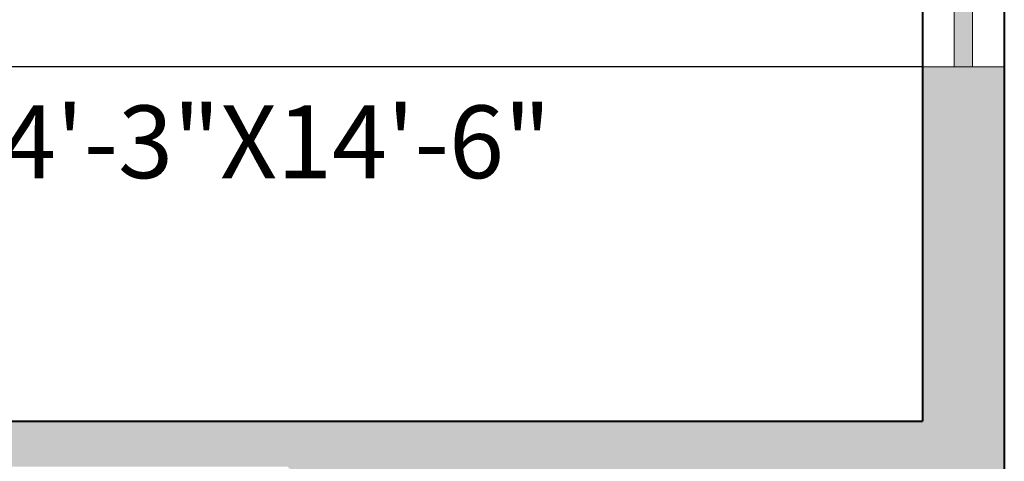
# Model space of a CAD drawing. Units: inches. Extents: x 2330 to 3943, y 1763 to 3461.
# Tile 32 of 40: x 3347 to 3456, y 2975 to 3024. Entities that reach past the tile are written whole.
import ezdxf

# ---------------------------------------------------------------- set-up
doc = ezdxf.new("R2010")
doc.units = ezdxf.units.IN
for name, color, linetype, lineweight in [('A-ANNO-DIMS', 2, 'Continuous', 18), ('A-AREA-IDEN', 7, 'Continuous', 18), ('A-GLAZ', 4, 'Continuous', 18), ('A-WALL', 7, 'Continuous', 40), ('A-WALL-PATT', 252, 'Continuous', 13)]:
    doc.layers.add(name, color=color, linetype=linetype, lineweight=lineweight)
doc.styles.get("Standard").update_dxf_attribs({"font": 'arial.ttf'})
doc.dimstyles.get("Standard").update_dxf_attribs({"dimtxt": 0.18, "dimasz": 0.18, "dimexe": 0.18, "dimexo": 0.0625, "dimgap": 0.09, "dimtad": 0, "dimtih": 1, "dimtoh": 1, "dimdec": 4, "dimzin": 0, "dimdsep": 46, "dimtxsty": 'Standard', "dimcen": 0.09, "dimadec": 0, "dimazin": 0, "dimtfac": 1, "dimtdec": 4, "dimtofl": 0, "dimtmove": 0, "dimatfit": 3, "dimfxl": 1, "dimtolj": 1, "dimtzin": 0, "dimarcsym": 0})

# ---------------------------------------------------------------- blocks, each defined once
blk = doc.blocks.new('WINDOW-96IN')
h = blk.add_hatch(color=256)
h.dxf.hatch_style = 1
h.paths.add_polyline_path([(5.5, 96), (3.5, 96), (3.5, 0), (5.5, 0)])
for p, q in [((0, 96), (9, 96)), ((3.5, 96), (3.5, 0)), ((5.5, 96), (5.5, 0)), ((0, 0), (9, 0))]:
    blk.add_line(p, q)
blk = doc.blocks.new('*D93')
at = {"layer": 'A-ANNO-DIMS', "color": 0, "lineweight": -2, "transparency": 16777216}
for p, q in [((3446.6, 3018.65), (2330.5, 3018.65)), ((2330.68, 3018.47), (2330.68, 2999.33)), ((2330.68, 2979.83), (2330.68, 2998.97)), ((3446.6, 2979.65), (2330.5, 2979.65))]:
    blk.add_line(p, q, dxfattribs=at)
at = {"layer": 'A-ANNO-DIMS', "color": 0, "transparency": 16777216}
for points in [[(2330.65, 3018.47), (2330.71, 3018.47), (2330.68, 3018.65)], [(2330.65, 2979.83), (2330.71, 2979.83), (2330.68, 2979.65)]]:
    blk.add_solid(points, dxfattribs=at)
at = {"layer": 'Defpoints', "color": 0, "transparency": 16777216}
for p in [(2330.68, 3018.65), (3446.66, 3018.65), (3446.66, 2979.65)]:
    blk.add_point(p, dxfattribs=at)
at = {"layer": 'A-ANNO-DIMS', "color": 0, "transparency": 16777216, "insert": (2330.68, 2999.15), "char_height": 0.18, "attachment_point": 5}
blk.add_mtext('\\A1;39', dxfattribs=at)

msp = doc.modelspace()

# ---------------------------------------------------------------- hatches: boundary and pattern name
at = {"layer": 'A-WALL-PATT'}
h = msp.add_hatch(color=256, dxfattribs=at)
h.dxf.hatch_style = 1
h.paths.add_polyline_path([(3241.6605, 2974.6524), (3376.7746, 2974.6524, -0.16828569), (3398.3014, 2935.4254), (3407.174, 2936.9344, 0.12044914), (3392.5913, 2970.6524), (3455.6605, 2970.6524), (3455.6605, 3018.6524), (3446.6605, 3018.6524), (3446.6605, 2979.6524), (3275.6605, 2979.6524), (3275.6605, 3018.6524), (3270.6605, 3018.6524), (3270.6605, 2979.6524), (3154.6605, 2979.6524), (3154.6605, 2918.1524), (3150.6605, 2918.1524), (3150.6605, 2913.1524), (3154.6605, 2913.1524), (3154.6605, 2863.6524), (3159.6605, 2863.6524), (3159.6605, 2867.6524), (3196.6605, 2867.6524), (3196.6605, 2872.6524), (3159.6605, 2872.6524), (3159.6605, 2974.6524), (3236.6605, 2974.6524), (3236.6605, 2906.6524), (3241.6605, 2906.6524)])

# ---------------------------------------------------------------- linework, layer by layer
at = {"layer": 'A-WALL'}
for p, q in [((3455.6605, 3162.6524), (3455.6605, 2970.6524)), ((3446.6605, 3153.6524), (3446.6605, 2979.6524)), ((3275.6605, 2979.6524), (3446.6605, 2979.6524))]:
    msp.add_line(p, q, dxfattribs=at)

# ---------------------------------------------------------------- block references
at = {"layer": 'A-GLAZ'}
msp.add_blockref('WINDOW-96IN', (3446.6605, 3018.6524), dxfattribs=at)

# ---------------------------------------------------------------- texts
at = {"layer": 'A-AREA-IDEN', "insert": (3339.1901, 3014.4043), "char_height": 8, "attachment_point": 1}
msp.add_mtext_dynamic_manual_height_columns('14\'-3"X14\'-6"', width=95.491359, gutter_width=12.5, heights=[0], dxfattribs=at)

# ---------------------------------------------------------------- dimensions: what is measured, and where the dimension line sits
at = {"layer": 'A-ANNO-DIMS'}
dim = msp.add_linear_dim(base=(2330.6824, 3018.6524), p1=(3446.6605, 2979.6524), p2=(3446.6605, 3018.6524), angle=90, dimstyle='Standard', override={"dimdec": 0, "dimlfac": 1, "dimrnd": 0, "dimzin": 0, "dimdsep": 46, "dimlunit": 2}, dxfattribs=at)
dim.commit()
dim.dimension.update_dxf_attribs({"geometry": '*D93', "text_midpoint": (2330.6824, 2999.1524)})

doc.saveas('drawing.dxf')
